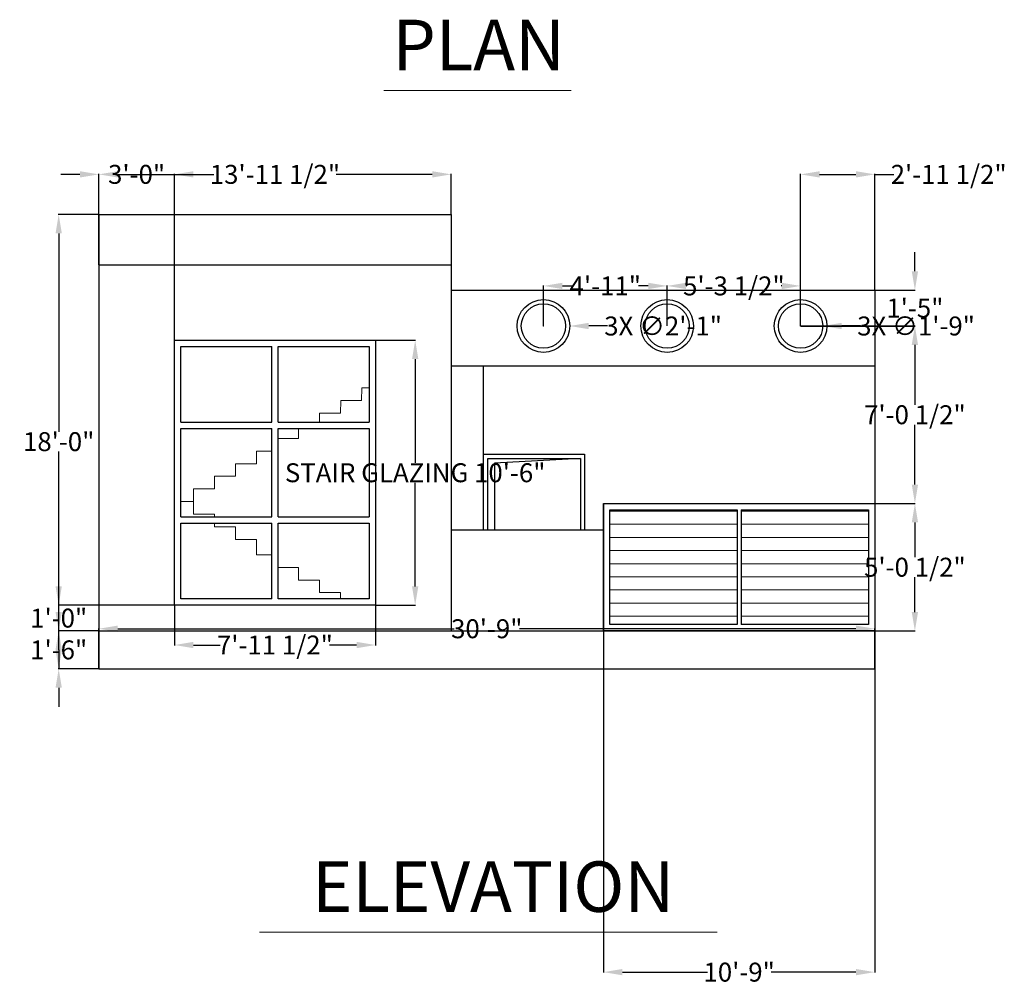
# Model space of a CAD drawing. Units: inches. Extents: x 68 to 1275, y 90 to 1276.
# Tile 1 of 6: x 128 to 596, y 94 to 552. Entities that reach past the tile are written whole.
import ezdxf

# ---------------------------------------------------------------- set-up
doc = ezdxf.new("R2010")
doc.units = ezdxf.units.IN
doc.header["$MEASUREMENT"] = 0
for name, color, linetype, lineweight in [('A-ANNO-TEXT', 7, 'Continuous', 18), ('A-DOOR-PATT', 8, 'Continuous', 13), ('A-ELEV', 7, 'Continuous', 25), ('DIM', 2, 'Continuous', 18), ('DOOR', 15, 'Continuous', 25), ('STAIRCASE', 40, 'Continuous', 18), ('WINDOW', 17, 'Continuous', 18)]:
    doc.layers.add(name, color=color, linetype=linetype, lineweight=lineweight)
doc.styles.get("Standard").update_dxf_attribs({"font": 'arial.ttf'})
doc.dimstyles.get("Standard").update_dxf_attribs({"dimtxt": 9, "dimasz": 9, "dimexe": 0.18, "dimexo": 0.0625, "dimgap": 0.09, "dimtad": 0, "dimtih": 1, "dimtoh": 1, "dimdec": 1, "dimzin": 0, "dimdsep": 46, "dimlunit": 3, "dimtxsty": 'Standard', "dimcen": 0.09, "dimadec": 0, "dimazin": 0, "dimtfac": 1, "dimtdec": 1, "dimtofl": 0, "dimtmove": 0, "dimatfit": 3, "dimfxl": 1, "dimtolj": 1, "dimtzin": 0, "dimarcsym": 0})

# ---------------------------------------------------------------- blocks, each defined once
blk = doc.blocks.new('WS')
at = {"layer": 'DOOR'}
for p, q in [((204.19, 360.98), (204.19, 396.98)), ((204.19, 396.98), (247.46, 396.98)), ((247.46, 360.98), (247.46, 396.98)), ((250.46, 396.98), (293.74, 396.98)), ((250.46, 360.98), (250.46, 396.98)), ((293.74, 396.98), (293.74, 360.98)), ((204.19, 360.98), (247.46, 360.98)), ((250.46, 360.98), (293.74, 360.98)), ((204.19, 315.98), (204.19, 357.98)), ((204.19, 357.98), (247.46, 357.98)), ((247.46, 315.98), (247.46, 357.98)), ((250.46, 315.98), (250.46, 357.98)), ((250.46, 357.98), (293.74, 357.98)), ((293.74, 357.98), (293.74, 315.98)), ((204.19, 315.98), (247.46, 315.98)), ((250.46, 315.98), (293.74, 315.98)), ((204.19, 276.98), (204.19, 312.98)), ((204.19, 312.98), (247.46, 312.98)), ((247.46, 276.98), (247.46, 312.98)), ((250.46, 276.98), (250.46, 312.98)), ((250.46, 312.98), (293.74, 312.98)), ((293.74, 312.98), (293.74, 276.98)), ((247.46, 276.98), (204.19, 276.98)), ((293.74, 276.98), (250.46, 276.98))]:
    blk.add_line(p, q, dxfattribs=at)
blk.add_lwpolyline([(201.19, 399.98), (296.74, 399.98), (296.74, 273.98), (201.19, 273.98)], close=True, dxfattribs=at)
blk = doc.blocks.new('FASCIA-ROUND-TRIM')
for radius in [12.52, 10.52]:
    blk.add_circle((0, 0), radius)
blk = doc.blocks.new('*D81')
at = {"layer": 'Defpoints', "color": 0, "transparency": 16777216}
for p in [(296.74, 399.98), (315.64, 399.98), (296.74, 273.98)]:
    blk.add_point(p, dxfattribs=at)
at = {"layer": 'DIM', "color": 0, "lineweight": -2, "transparency": 16777216}
for p, q in [((296.8, 399.98), (315.82, 399.98)), ((315.64, 390.98), (315.64, 341.72)), ((315.64, 282.98), (315.64, 332.24)), ((296.8, 273.98), (315.82, 273.98))]:
    blk.add_line(p, q, dxfattribs=at)
at = {"layer": 'DIM', "color": 0, "transparency": 16777216}
for points in [[(314.14, 390.98), (317.14, 390.98), (315.64, 399.98)], [(314.14, 282.98), (317.14, 282.98), (315.64, 273.98)]]:
    blk.add_solid(points, dxfattribs=at)
at = {"layer": 'DIM', "color": 0, "transparency": 16777216, "insert": (315.64, 336.98), "char_height": 9, "attachment_point": 5}
blk.add_mtext('\\A1;STAIR GLAZING 10\'-6"', dxfattribs=at)
blk = doc.blocks.new('*D82')
at = {"layer": 'Defpoints', "color": 0, "transparency": 16777216}
for p in [(201.19, 273.98), (296.74, 273.98), (296.74, 255.08)]:
    blk.add_point(p, dxfattribs=at)
at = {"layer": 'DIM', "color": 0, "lineweight": -2, "transparency": 16777216}
for p, q in [((201.19, 273.92), (201.19, 254.9)), ((296.74, 273.92), (296.74, 254.9)), ((210.19, 255.08), (222.97, 255.08)), ((287.74, 255.08), (274.96, 255.08))]:
    blk.add_line(p, q, dxfattribs=at)
at = {"layer": 'DIM', "color": 0, "transparency": 16777216}
for points in [[(210.19, 256.58), (210.19, 253.58), (201.19, 255.08)], [(287.74, 256.58), (287.74, 253.58), (296.74, 255.08)]]:
    blk.add_solid(points, dxfattribs=at)
at = {"layer": 'DIM', "color": 0, "transparency": 16777216, "insert": (248.96, 255.08), "char_height": 9, "attachment_point": 5}
blk.add_mtext('\\A1;7\'-11 1/2"', dxfattribs=at)
blk = doc.blocks.new('*D86')
at = {"layer": 'Defpoints', "color": 0, "transparency": 16777216}
for p in [(534.19, 262.82), (165.19, 243.77), (534.19, 243.77)]:
    blk.add_point(p, dxfattribs=at)
at = {"layer": 'DIM', "color": 0, "lineweight": -2, "transparency": 16777216}
for p, q in [((165.19, 243.83), (165.19, 263)), ((174.19, 262.82), (334.15, 262.82)), ((525.19, 262.82), (365.24, 262.82)), ((534.19, 243.83), (534.19, 263))]:
    blk.add_line(p, q, dxfattribs=at)
at = {"layer": 'DIM', "color": 0, "transparency": 16777216}
for points in [[(174.19, 264.32), (174.19, 261.32), (165.19, 262.82)], [(525.19, 264.32), (525.19, 261.32), (534.19, 262.82)]]:
    blk.add_solid(points, dxfattribs=at)
at = {"layer": 'DIM', "color": 0, "transparency": 16777216, "insert": (349.69, 262.82), "char_height": 9, "attachment_point": 5}
blk.add_mtext('\\A1;30\'-9"', dxfattribs=at)
blk = doc.blocks.new('*D87')
at = {"layer": 'Defpoints', "color": 0, "transparency": 16777216}
for p in [(146.14, 459.77), (165.19, 459.77), (165.19, 243.77)]:
    blk.add_point(p, dxfattribs=at)
at = {"layer": 'DIM', "color": 0, "lineweight": -2, "transparency": 16777216}
for p, q in [((165.13, 459.77), (145.96, 459.77)), ((146.14, 450.77), (146.14, 356.46)), ((146.14, 252.77), (146.14, 347.09)), ((165.13, 243.77), (145.96, 243.77))]:
    blk.add_line(p, q, dxfattribs=at)
at = {"layer": 'DIM', "color": 0, "transparency": 16777216}
for points in [[(144.64, 450.77), (147.64, 450.77), (146.14, 459.77)], [(144.64, 252.77), (147.64, 252.77), (146.14, 243.77)]]:
    blk.add_solid(points, dxfattribs=at)
at = {"layer": 'DIM', "color": 0, "transparency": 16777216, "insert": (146.14, 351.77), "char_height": 9, "attachment_point": 5}
blk.add_mtext('\\A1;18\'-0"', dxfattribs=at)
blk = doc.blocks.new('*D88')
at = {"layer": 'Defpoints', "color": 0, "transparency": 16777216}
for p in [(332.74, 478.82), (165.19, 459.77), (332.74, 459.77)]:
    blk.add_point(p, dxfattribs=at)
at = {"layer": 'DIM', "color": 0, "lineweight": -2, "transparency": 16777216}
for p, q in [((165.19, 459.83), (165.19, 479)), ((174.19, 478.82), (219.86, 478.82)), ((323.74, 478.82), (278.07, 478.82)), ((332.74, 459.83), (332.74, 479))]:
    blk.add_line(p, q, dxfattribs=at)
at = {"layer": 'DIM', "color": 0, "transparency": 16777216}
for points in [[(174.19, 480.32), (174.19, 477.32), (165.19, 478.82)], [(323.74, 480.32), (323.74, 477.32), (332.74, 478.82)]]:
    blk.add_solid(points, dxfattribs=at)
at = {"layer": 'DIM', "color": 0, "transparency": 16777216, "insert": (248.96, 478.82), "char_height": 9, "attachment_point": 5}
blk.add_mtext('\\A1;13\'-11 1/2"', dxfattribs=at)
blk = doc.blocks.new('*D89')
at = {"layer": 'Defpoints', "color": 0, "transparency": 16777216}
for p in [(498.9, 406.74), (553.24, 406.74), (534.19, 322.39)]:
    blk.add_point(p, dxfattribs=at)
at = {"layer": 'DIM', "color": 0, "lineweight": -2, "transparency": 16777216}
for p, q in [((498.96, 406.74), (553.42, 406.74)), ((553.24, 397.74), (553.24, 369.31)), ((553.24, 331.39), (553.24, 359.82)), ((534.25, 322.39), (553.42, 322.39))]:
    blk.add_line(p, q, dxfattribs=at)
at = {"layer": 'DIM', "color": 0, "transparency": 16777216}
for points in [[(551.74, 397.74), (554.74, 397.74), (553.24, 406.74)], [(551.74, 331.39), (554.74, 331.39), (553.24, 322.39)]]:
    blk.add_solid(points, dxfattribs=at)
at = {"layer": 'DIM', "color": 0, "transparency": 16777216, "insert": (553.24, 364.56), "char_height": 9, "attachment_point": 5}
blk.add_mtext('\\A1;7\'-0 1/2"', dxfattribs=at)
blk = doc.blocks.new('*D90')
at = {"layer": 'Defpoints', "color": 0, "transparency": 16777216}
for p in [(146.142058, 261.770671), (165.192058, 261.770671), (165.192058, 243.770671)]:
    blk.add_point(p, dxfattribs=at)
at = {"layer": 'DIM', "color": 0, "lineweight": -2, "transparency": 16777216}
for p, q in [((146.142058, 270.770671), (146.142058, 279.770671)), ((165.129558, 261.770671), (145.962058, 261.770671)), ((165.129558, 243.770671), (145.962058, 243.770671)), ((146.142058, 234.770671), (146.142058, 225.770671))]:
    blk.add_line(p, q, dxfattribs=at)
at = {"layer": 'DIM', "color": 0, "transparency": 16777216}
for points in [[(144.642058, 270.770671), (147.642058, 270.770671), (146.142058, 261.770671)], [(144.642058, 234.770671), (147.642058, 234.770671), (146.142058, 243.770671)]]:
    blk.add_solid(points, dxfattribs=at)
at = {"layer": 'DIM', "color": 0, "transparency": 16777216, "insert": (146.142058, 252.770671), "char_height": 9, "attachment_point": 5}
blk.add_mtext('\\A1;1\'-6"', dxfattribs=at)
blk = doc.blocks.new('*D91')
at = {"layer": 'Defpoints', "color": 0, "transparency": 16777216}
for p in [(405.19, 261.77), (534.19, 261.77), (534.19, 99.58)]:
    blk.add_point(p, dxfattribs=at)
at = {"layer": 'DIM', "color": 0, "lineweight": -2, "transparency": 16777216}
for p, q in [((405.19, 261.71), (405.19, 99.4)), ((534.19, 261.71), (534.19, 99.4)), ((414.19, 99.58), (454.57, 99.58)), ((525.19, 99.58), (484.82, 99.58))]:
    blk.add_line(p, q, dxfattribs=at)
at = {"layer": 'DIM', "color": 0, "transparency": 16777216}
for points in [[(414.19, 101.08), (414.19, 98.08), (405.19, 99.58)], [(525.19, 101.08), (525.19, 98.08), (534.19, 99.58)]]:
    blk.add_solid(points, dxfattribs=at)
at = {"layer": 'DIM', "color": 0, "transparency": 16777216, "insert": (469.69, 99.58), "char_height": 9, "attachment_point": 5}
blk.add_mtext('\\A1;10\'-9"', dxfattribs=at)
blk = doc.blocks.new('*D92')
at = {"layer": 'Defpoints', "color": 0, "transparency": 16777216}
for p in [(201.192058, 478.820671), (165.192058, 435.770671), (201.192058, 399.981388)]:
    blk.add_point(p, dxfattribs=at)
at = {"layer": 'DIM', "color": 0, "lineweight": -2, "transparency": 16777216}
for p, q in [((156.192058, 478.820671), (147.192058, 478.820671)), ((165.192058, 435.833171), (165.192058, 479.000671)), ((201.192058, 400.043888), (201.192058, 479.000671)), ((210.192058, 478.820671), (219.192058, 478.820671))]:
    blk.add_line(p, q, dxfattribs=at)
at = {"layer": 'DIM', "color": 0, "transparency": 16777216}
for points in [[(156.192058, 480.320671), (156.192058, 477.320671), (165.192058, 478.820671)], [(210.192058, 480.320671), (210.192058, 477.320671), (201.192058, 478.820671)]]:
    blk.add_solid(points, dxfattribs=at)
at = {"layer": 'DIM', "color": 0, "transparency": 16777216, "insert": (183.192058, 478.820671), "char_height": 9, "attachment_point": 5}
blk.add_mtext('\\A1;3\'-0"', dxfattribs=at)
blk = doc.blocks.new('*D93')
at = {"layer": 'Defpoints', "color": 0, "transparency": 16777216}
for p in [(146.14, 273.98), (201.19, 273.98), (165.19, 261.77)]:
    blk.add_point(p, dxfattribs=at)
at = {"layer": 'DIM', "color": 0, "lineweight": -2, "transparency": 16777216}
for p, q in [((146.14, 282.98), (146.14, 291.98)), ((201.13, 273.98), (145.96, 273.98)), ((165.13, 261.77), (145.96, 261.77)), ((146.14, 252.77), (146.14, 243.77))]:
    blk.add_line(p, q, dxfattribs=at)
at = {"layer": 'DIM', "color": 0, "transparency": 16777216}
for points in [[(144.64, 282.98), (147.64, 282.98), (146.14, 273.98)], [(144.64, 252.77), (147.64, 252.77), (146.14, 261.77)]]:
    blk.add_solid(points, dxfattribs=at)
at = {"layer": 'DIM', "color": 0, "transparency": 16777216, "insert": (146.14, 267.88), "char_height": 9, "attachment_point": 5}
blk.add_mtext('\\A1;1\'-0"', dxfattribs=at)
blk = doc.blocks.new('*D94')
at = {"layer": 'Defpoints', "color": 0, "transparency": 16777216}
for p in [(534.19, 322.39), (553.24, 322.39), (534.19, 261.77)]:
    blk.add_point(p, dxfattribs=at)
at = {"layer": 'DIM', "color": 0, "lineweight": -2, "transparency": 16777216}
for p, q in [((534.25, 322.39), (553.42, 322.39)), ((553.24, 313.39), (553.24, 296.82)), ((553.24, 270.77), (553.24, 287.34)), ((534.25, 261.77), (553.42, 261.77))]:
    blk.add_line(p, q, dxfattribs=at)
at = {"layer": 'DIM', "color": 0, "transparency": 16777216}
for points in [[(551.74, 313.39), (554.74, 313.39), (553.24, 322.39)], [(551.74, 270.77), (554.74, 270.77), (553.24, 261.77)]]:
    blk.add_solid(points, dxfattribs=at)
at = {"layer": 'DIM', "color": 0, "transparency": 16777216, "insert": (553.24, 292.08), "char_height": 9, "attachment_point": 5}
blk.add_mtext('\\A1;5\'-0 1/2"', dxfattribs=at)
blk = doc.blocks.new('*D95')
at = {"layer": 'Defpoints', "color": 0, "transparency": 16777216}
for p in [(435.45, 425.79), (376.62, 406.74), (435.45, 406.74)]:
    blk.add_point(p, dxfattribs=at)
at = {"layer": 'DIM', "color": 0, "lineweight": -2, "transparency": 16777216}
for p, q in [((376.62, 406.8), (376.62, 425.97)), ((385.62, 425.79), (390.31, 425.79)), ((426.45, 425.79), (421.77, 425.79)), ((435.45, 406.8), (435.45, 425.97))]:
    blk.add_line(p, q, dxfattribs=at)
at = {"layer": 'DIM', "color": 0, "transparency": 16777216}
for points in [[(385.62, 427.29), (385.62, 424.29), (376.62, 425.79)], [(426.45, 427.29), (426.45, 424.29), (435.45, 425.79)]]:
    blk.add_solid(points, dxfattribs=at)
at = {"layer": 'DIM', "color": 0, "transparency": 16777216, "insert": (406.04, 425.79), "char_height": 9, "attachment_point": 5}
blk.add_mtext('\\A1;4\'-11"', dxfattribs=at)
blk = doc.blocks.new('*D96')
at = {"layer": 'Defpoints', "color": 0, "transparency": 16777216}
for p in [(498.9, 425.79), (435.45, 406.74), (498.9, 406.74)]:
    blk.add_point(p, dxfattribs=at)
at = {"layer": 'DIM', "color": 0, "lineweight": -2, "transparency": 16777216}
for p, q in [((435.45, 406.8), (435.45, 425.97)), ((444.45, 425.79), (444.64, 425.79)), ((489.9, 425.79), (489.71, 425.79)), ((498.9, 406.8), (498.9, 425.97))]:
    blk.add_line(p, q, dxfattribs=at)
at = {"layer": 'DIM', "color": 0, "transparency": 16777216}
for points in [[(444.45, 427.29), (444.45, 424.29), (435.45, 425.79)], [(489.9, 427.29), (489.9, 424.29), (498.9, 425.79)]]:
    blk.add_solid(points, dxfattribs=at)
at = {"layer": 'DIM', "color": 0, "transparency": 16777216, "insert": (467.18, 425.79), "char_height": 9, "attachment_point": 5}
blk.add_mtext('\\A1;5\'-3 1/2"', dxfattribs=at)
blk = doc.blocks.new('*D97')
at = {"layer": 'Defpoints', "color": 0, "transparency": 16777216}
for p in [(534.19, 478.82), (534.19, 423.77), (498.9, 406.74)]:
    blk.add_point(p, dxfattribs=at)
at = {"layer": 'DIM', "color": 0, "lineweight": -2, "transparency": 16777216}
for p, q in [((498.9, 406.8), (498.9, 479)), ((507.9, 478.82), (525.19, 478.82)), ((534.19, 423.83), (534.19, 479)), ((534.19, 478.82), (543.19, 478.82))]:
    blk.add_line(p, q, dxfattribs=at)
at = {"layer": 'DIM', "color": 0, "transparency": 16777216}
for points in [[(507.9, 480.32), (507.9, 477.32), (498.9, 478.82)], [(525.19, 480.32), (525.19, 477.32), (534.19, 478.82)]]:
    blk.add_solid(points, dxfattribs=at)
at = {"layer": 'DIM', "color": 0, "transparency": 16777216, "insert": (569.3, 478.82), "char_height": 9, "attachment_point": 5}
blk.add_mtext('\\A1;2\'-11 1/2"', dxfattribs=at)
blk = doc.blocks.new('*D98')
at = {"layer": 'Defpoints', "color": 0, "transparency": 16777216}
for p in [(534.192058, 423.770671), (553.242058, 423.770671), (498.898193, 406.737347)]:
    blk.add_point(p, dxfattribs=at)
at = {"layer": 'DIM', "color": 0, "lineweight": -2, "transparency": 16777216}
for p, q in [((553.242058, 432.770671), (553.242058, 441.770671)), ((534.254558, 423.770671), (553.422058, 423.770671)), ((498.960693, 406.737347), (553.422058, 406.737347)), ((553.242058, 397.737347), (553.242058, 388.737347))]:
    blk.add_line(p, q, dxfattribs=at)
at = {"layer": 'DIM', "color": 0, "transparency": 16777216}
for points in [[(551.742058, 432.770671), (554.742058, 432.770671), (553.242058, 423.770671)], [(551.742058, 397.737347), (554.742058, 397.737347), (553.242058, 406.737347)]]:
    blk.add_solid(points, dxfattribs=at)
at = {"layer": 'DIM', "color": 0, "transparency": 16777216, "insert": (553.242058, 415.254009), "char_height": 9, "attachment_point": 5}
blk.add_mtext('\\A1;1\'-5"', dxfattribs=at)
blk = doc.blocks.new('*D114')
at = {"layer": 'Defpoints', "color": 0, "transparency": 16777216}
for p in [(364.1, 406.74), (389.14, 406.74)]:
    blk.add_point(p, dxfattribs=at)
at = {"layer": 'DIM', "color": 0, "lineweight": -2, "transparency": 16777216}
for p, q in [((376.53, 406.74), (376.71, 406.74)), ((376.62, 406.65), (376.62, 406.83)), ((407.14, 406.74), (398.14, 406.74))]:
    blk.add_line(p, q, dxfattribs=at)
at = {"layer": 'DIM', "color": 0, "transparency": 16777216}
blk.add_solid([(398.14, 408.24), (398.14, 405.24), (389.14, 406.74)], dxfattribs=at)
at = {"layer": 'DIM', "color": 0, "transparency": 16777216, "insert": (433.52, 406.74), "char_height": 9, "attachment_point": 5}
blk.add_mtext('\\A1;3X ∅2\'-1"', dxfattribs=at)
blk = doc.blocks.new('*D115')
at = {"layer": 'Defpoints', "color": 0, "transparency": 16777216}
for p in [(488.38, 406.74), (509.42, 406.74)]:
    blk.add_point(p, dxfattribs=at)
at = {"layer": 'DIM', "color": 0, "lineweight": -2, "transparency": 16777216}
for p, q in [((498.81, 406.74), (498.99, 406.74)), ((498.9, 406.65), (498.9, 406.83)), ((527.42, 406.74), (518.42, 406.74))]:
    blk.add_line(p, q, dxfattribs=at)
at = {"layer": 'DIM', "color": 0, "transparency": 16777216}
blk.add_solid([(518.42, 408.24), (518.42, 405.24), (509.42, 406.74)], dxfattribs=at)
at = {"layer": 'DIM', "color": 0, "transparency": 16777216, "insert": (553.79, 406.74), "char_height": 9, "attachment_point": 5}
blk.add_mtext('\\A1;3X ∅1\'-9"', dxfattribs=at)

msp = doc.modelspace()

# ---------------------------------------------------------------- hatches: boundary and pattern name
at = {"layer": 'A-DOOR-PATT', "transparency": 33554531}
h = msp.add_hatch(dxfattribs=at)
h.set_pattern_fill('LINE', color=256, scale=50)
h.paths.add_polyline_path([(468.69, 319.39), (408.19, 319.39), (408.19, 264.77), (468.69, 264.77)])
h.paths.add_polyline_path([(531.19, 319.39), (470.69, 319.39), (470.69, 264.77), (531.19, 264.77)])

# ---------------------------------------------------------------- linework, layer by layer
at = {"layer": 'A-ANNO-TEXT'}
for p, q in [((300.67, 518.76), (389.82, 518.76)), ((241.59, 118.63), (459.16, 118.63))]:
    msp.add_line(p, q, dxfattribs=at)
at = {"layer": 'A-ELEV'}
for p, q in [((165.19, 459.77), (332.74, 459.77)), ((165.19, 459.77), (165.19, 243.77)), ((332.74, 459.77), (332.74, 261.77)), ((165.19, 435.77), (332.74, 435.77)), ((332.74, 423.77), (534.19, 423.77)), ((534.19, 423.77), (534.19, 243.77)), ((332.74, 387.77), (534.19, 387.77)), ((348.19, 309.77), (348.19, 387.77)), ((332.74, 309.77), (405.19, 309.77)), ((165.19, 261.77), (407.28, 261.77)), ((405.19, 261.77), (534.19, 261.77)), ((165.19, 243.77), (534.19, 243.77))]:
    msp.add_line(p, q, dxfattribs=at)
at = {"layer": 'DOOR'}
for p, q in [((348.19, 309.77), (348.19, 345.77)), ((348.19, 345.77), (396.19, 345.77)), ((350.19, 343.77), (394.19, 343.77)), ((350.19, 309.77), (350.19, 343.77)), ((394.19, 343.77), (353.43, 341.48)), ((394.19, 343.77), (394.19, 309.77)), ((396.19, 345.77), (396.19, 309.77)), ((353.43, 341.48), (353.43, 309.77)), ((405.19, 322.39), (405.19, 261.77)), ((405.19, 322.39), (534.19, 322.39)), ((468.69, 319.39), (468.69, 264.77)), ((470.69, 319.39), (470.69, 264.77))]:
    msp.add_line(p, q, dxfattribs=at)
msp.add_lwpolyline([(405.19, 322.39), (534.19, 322.39), (534.19, 261.77), (405.19, 261.77)], close=True, dxfattribs=at)
for points in [[(468.69, 264.77), (408.19, 264.77), (408.19, 319.39), (468.69, 319.39)], [(470.69, 319.39), (531.19, 319.39), (531.19, 264.77), (470.69, 264.77)]]:
    msp.add_lwpolyline(points, dxfattribs=at)
at = {"layer": 'STAIRCASE'}
for p, q in [((290.19, 371.28), (290.22, 377.28)), ((290.22, 377.28), (293.74, 377.28)), ((280.19, 365.28), (280.22, 371.28)), ((280.22, 371.28), (290.19, 371.28)), ((270.2, 360.98), (270.22, 365.28)), ((270.22, 365.28), (280.19, 365.28)), ((260.19, 353.28), (260.22, 357.98)), ((250.46, 353.28), (260.19, 353.28)), ((240.19, 341.28), (240.22, 347.28)), ((240.22, 347.28), (247.46, 347.28)), ((230.19, 335.28), (230.22, 341.28)), ((230.22, 341.28), (240.19, 341.28)), ((220.19, 329.28), (220.22, 335.28)), ((220.22, 335.28), (230.19, 335.28)), ((210.19, 323.28), (210.22, 329.28)), ((210.22, 329.28), (220.19, 329.28)), ((210.19, 323.28), (204.19, 323.28)), ((210.19, 317.28), (210.19, 323.28)), ((220.19, 317.28), (210.19, 317.28)), ((220.19, 315.98), (220.19, 317.28)), ((220.19, 311.28), (220.19, 312.98)), ((230.19, 311.28), (220.19, 311.28)), ((230.19, 305.28), (230.19, 311.28)), ((240.19, 305.28), (230.19, 305.28)), ((240.19, 297.98), (240.19, 305.28)), ((247.46, 297.98), (240.19, 297.98)), ((260.19, 291.98), (250.46, 291.98)), ((260.19, 285.98), (260.19, 291.98)), ((270.19, 285.98), (260.19, 285.98)), ((270.19, 279.98), (270.19, 285.98)), ((280.19, 279.98), (270.19, 279.98)), ((280.19, 276.98), (280.19, 279.98))]:
    msp.add_line(p, q, dxfattribs=at)

# ---------------------------------------------------------------- block references
at = {"layer": 'A-ELEV'}
for p in [(376.62, 406.74), (435.45, 406.74), (498.9, 406.74)]:
    msp.add_blockref('FASCIA-ROUND-TRIM', p, dxfattribs=at)
at = {"layer": 'WINDOW'}
msp.add_blockref('WS', (0, 0), dxfattribs=at)

# ---------------------------------------------------------------- texts
at = {"layer": 'A-ANNO-TEXT', "char_height": 24, "attachment_point": 2}
for s, width, insert in [('PLAN', 128.8568, (345.77, 552.35)), ('ELEVATION', 255.8943, (352.67, 152.22))]:
    msp.add_mtext_dynamic_manual_height_columns(s, width=width, gutter_width=1, heights=[0], dxfattribs=dict(at, insert=insert))

# ---------------------------------------------------------------- dimensions: what is measured, and where the dimension line sits
at = {"layer": 'DIM'}
for base, p1, p2, picture, middle in [((332.7361, 478.8207), (165.1921, 459.7707), (332.7361, 459.7707), '*D88', (248.9641, 478.8207)), ((534.19, 478.82), (498.9, 406.74), (534.19, 423.77), '*D97', (569.3, 478.82)), ((201.19, 478.82), (165.19, 435.77), (201.19, 399.98), '*D92', (183.19, 478.82)), ((498.8982, 425.7873), (435.4524, 406.7373), (498.8982, 406.7373), '*D96', (467.1753, 425.7873)), ((435.45, 425.79), (376.62, 406.74), (435.45, 406.74), '*D95', (406.04, 425.79)), ((296.7361, 255.0814), (201.1921, 273.9814), (296.7361, 273.9814), '*D82', (248.9641, 255.0814)), ((534.19, 262.82), (165.19, 243.77), (534.19, 243.77), '*D86', (349.69, 262.82)), ((534.19, 99.58), (405.19, 261.77), (534.19, 261.77), '*D91', (469.69, 99.58))]:
    dim = msp.add_linear_dim(base=base, p1=p1, p2=p2, dimstyle='Standard', override={"dimdec": 1, "dimlfac": 1, "dimrnd": 0, "dimzin": 1, "dimdsep": 46, "dimlunit": 4, "dimfrac": 2}, dxfattribs=at)
    dim.commit()
    dim.dimension.update_dxf_attribs({"geometry": picture, "text_midpoint": middle})
for base, p1, p2, picture, middle in [((146.14, 459.77), (165.19, 243.77), (165.19, 459.77), '*D87', (146.14, 351.77)), ((553.24, 423.77), (498.9, 406.74), (534.19, 423.77), '*D98', (553.24, 415.25)), ((553.2421, 406.7373), (534.1921, 322.3881), (498.8982, 406.7373), '*D89', (553.2421, 364.5627)), ((553.24, 322.39), (534.19, 261.77), (534.19, 322.39), '*D94', (553.24, 292.08)), ((146.14, 273.98), (165.19, 261.77), (201.19, 273.98), '*D93', (146.14, 267.88)), ((146.14, 261.77), (165.19, 243.77), (165.19, 261.77), '*D90', (146.14, 252.77))]:
    dim = msp.add_linear_dim(base=base, p1=p1, p2=p2, angle=90, dimstyle='Standard', override={"dimdec": 1, "dimlfac": 1, "dimrnd": 0, "dimzin": 1, "dimdsep": 46, "dimlunit": 4, "dimfrac": 2}, dxfattribs=at)
    dim.commit()
    dim.dimension.update_dxf_attribs({"geometry": picture, "text_midpoint": middle})
dim = msp.add_diameter_dim_2p(p1=(364.1, 406.74), p2=(389.14, 406.74), text='3X <>', dimstyle='Standard', override={"dimdec": 1, "dimlfac": 1, "dimrnd": 0, "dimzin": 1, "dimdsep": 46, "dimlunit": 4, "dimfrac": 2}, dxfattribs=at)
dim.commit()
dim.dimension.update_dxf_attribs({"geometry": '*D114', "text_midpoint": (407.14, 406.74), "dimtype": 163})
dim = msp.add_diameter_dim_2p(p1=(488.38, 406.74), p2=(509.42, 406.74), text='3X <>', dimstyle='Standard', override={"dimdec": 1, "dimlfac": 1, "dimrnd": 0, "dimzin": 1, "dimdsep": 46, "dimlunit": 4, "dimfrac": 2}, dxfattribs=at)
dim.commit()
dim.dimension.update_dxf_attribs({"geometry": '*D115', "text_midpoint": (527.42, 406.74)})
dim = msp.add_linear_dim(base=(315.64, 399.98), p1=(296.74, 273.98), p2=(296.74, 399.98), angle=90, text='STAIR GLAZING <>', dimstyle='Standard', override={"dimdec": 1, "dimlfac": 1, "dimrnd": 0, "dimzin": 1, "dimdsep": 46, "dimlunit": 4, "dimfrac": 2}, dxfattribs=at)
dim.commit()
dim.dimension.update_dxf_attribs({"geometry": '*D81', "text_midpoint": (315.64, 336.98)})

doc.saveas('drawing.dxf')
